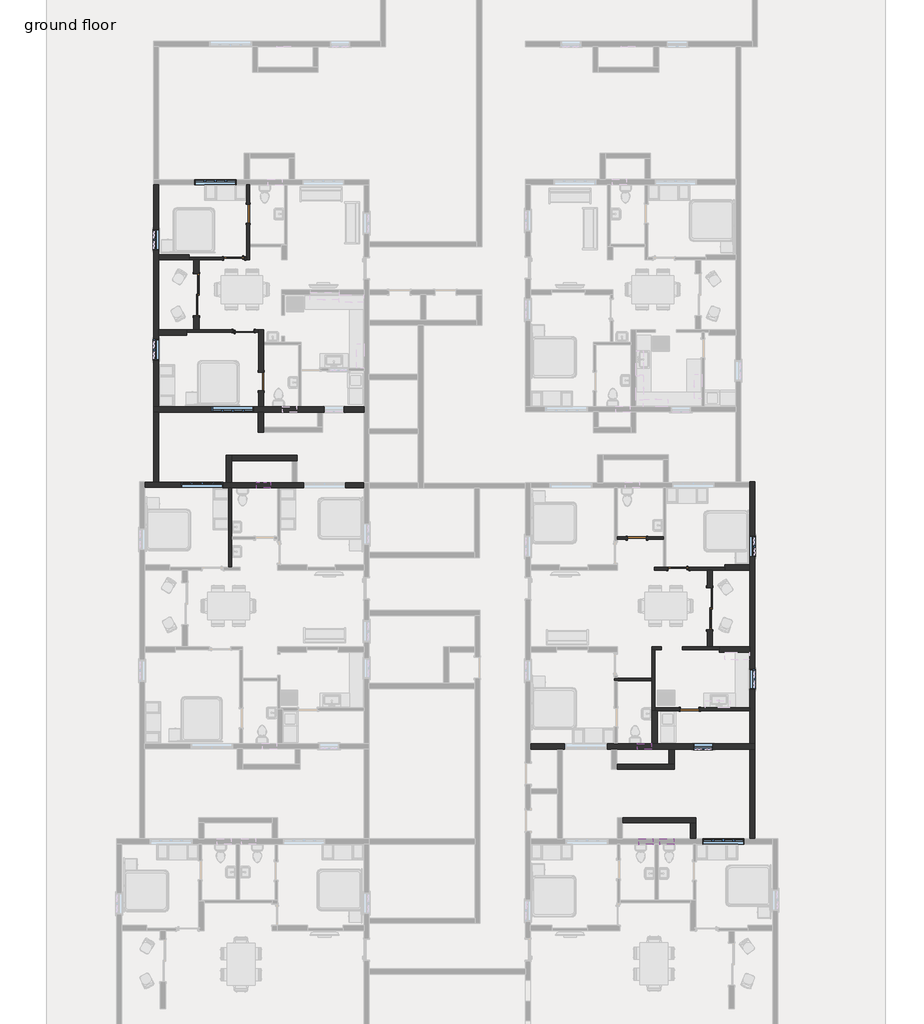
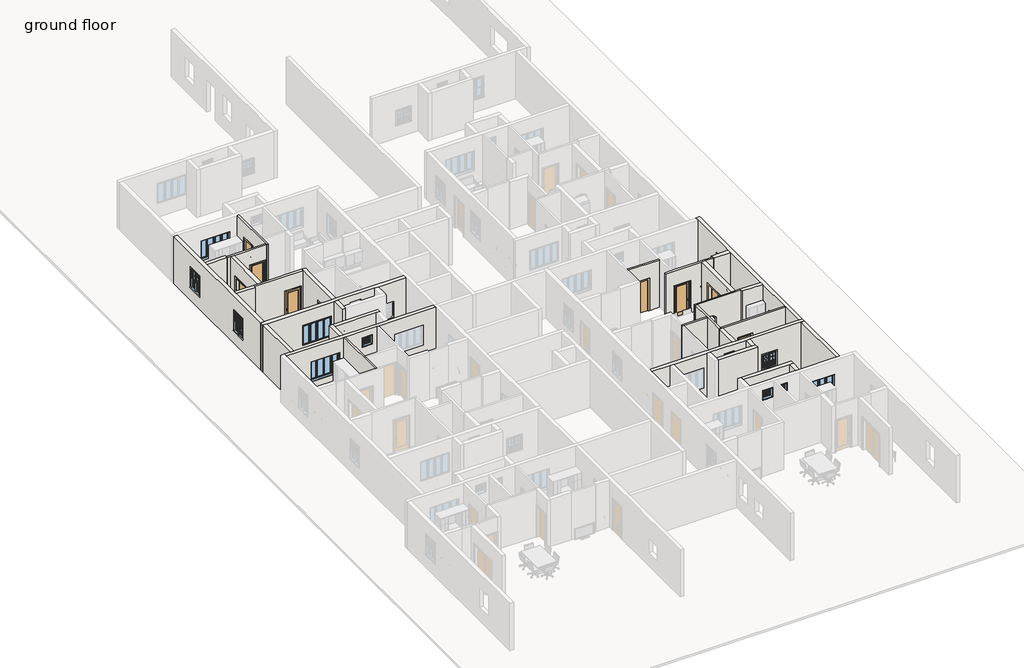
# One storey, part 4 of 16: 32 walls, 13 windows, 9 doors.
# Revit data of these elements (continued)
# Element 42 (IfcWindow, "Window-Casement-Double-Awning : 34\" x 36\"")
#   Mark = "76"
#   Window Inset = 0' - 0"
#   Interior Wall Closure = 0' - 2 1/4"
#   Frame Extension = 0' - 0 1/4"
#   Exterior Wall Closure = 0' - 1 1/4"
#   Interior Trim Visibility = yes
#   Exterior Trim Visibility = yes
#   Phase Created = New Construction
#   Materials on its faces: "Wood - Stained", "Glass", "Clad - White"
# Element 43 (IfcWindow, "Window-Casement-Double-Awning : 34\" x 36\"")
#   Mark = "77"
#   Window Inset = 0' - 0"
#   Interior Wall Closure = 0' - 2 1/4"
#   Frame Extension = 0' - 0 1/4"
#   Exterior Wall Closure = 0' - 1 1/4"
#   Interior Trim Visibility = yes
#   Exterior Trim Visibility = yes
#   Phase Created = New Construction
#   Materials on its faces: "Wood - Stained", "Glass", "Clad - White"
# Element 44 (IfcWindow, "Window-Casement-Multi-Sash-Horizontal : 72\" x 53\"")
#   Mark = "30"
#   Window Inset = 0' - 0 5/8"
#   Frame Gap 3 = 0' - 1 83/128"
#   Frame Gap 2 = 0' - 0 5/8"
#   Phase Created = New Construction
#   Materials on its faces: "Metal - Aluminum", "Glass"
# Element 45 (IfcWindow, "Window-Casement-Multi-Sash-Horizontal : 72\" x 53\"")
#   Mark = "35"
#   Window Inset = 0' - 0 5/8"
#   Frame Gap 3 = 0' - 1 83/128"
#   Frame Gap 2 = 0' - 0 5/8"
#   Phase Created = New Construction
#   Materials on its faces: "Metal - Aluminum", "Glass"
# Element 46 (IfcWindow, "Window-Casement-Multi-Sash-Horizontal : 72\" x 53\"")
#   Mark = "37"
#   Window Inset = 0' - 0 5/8"
#   Frame Gap 3 = 0' - 1 83/128"
#   Frame Gap 2 = 0' - 0 5/8"
#   Phase Created = New Construction
#   Materials on its faces: "Metal - Aluminum", "Glass"
# Element 47 (IfcWindow, "Window-Casement-Multi-Sash-Horizontal : 72\" x 53\"")
#   Mark = "38"
#   Window Inset = 0' - 0 5/8"
#   Frame Gap 3 = 0' - 1 83/128"
#   Frame Gap 2 = 0' - 0 5/8"
#   Phase Created = New Construction
#   Materials on its faces: "Metal - Aluminum", "Glass"
# Element 48 (IfcWindow, "Window-Louvers : 24\" x 24\"")
#   Mark = "99"
#   Blade Width = 1' - 10 1/2"
#   Phase Created = New Construction
#   Materials on its faces: "Birch"
# Element 49 (IfcWindow, "Window-Louvers : 24\" x 24\"")
#   Mark = "100"
#   Blade Width = 1' - 10 1/2"
#   Phase Created = New Construction
#   Materials on its faces: "Birch"
# Element 50 (IfcWindow, "Window-Louvers : 24\" x 24\"")
#   Mark = "101"
#   Blade Width = 1' - 10 1/2"
#   Phase Created = New Construction
#   Materials on its faces: "Birch"
# Element 51 (IfcWindow, "Window-Louvers : 24\" x 24\"")
#   Mark = "107"
#   Blade Width = 1' - 10 1/2"
#   Phase Created = New Construction
#   Materials on its faces: "Birch"
# Element 52 (IfcWindow, "Window-Single-Hung-Double : 36\" x 52\"")
#   Mark = "50"
#   Window Inset = 0' - 0"
#   Interior Wall Closure = 0' - 1 1/2"
#   Frame Extension = 0' - 1 1/4"
#   Exterior Wall Closure = 0' - 0 1/2"
#   Interior Trim Visibility = yes
#   Indicator Visibility = yes
#   Exterior Trim Visibility = yes
#   Phase Created = New Construction
#   Materials on its faces: "Wood - Stained", "Glass", "Clad - White"
# Element 53 (IfcWindow, "Window-Single-Hung-Double : 36\" x 52\"")
#   Mark = "61"
#   Window Inset = 0' - 0"
#   Interior Wall Closure = 0' - 1 1/2"
#   Frame Extension = 0' - 1 1/4"
#   Exterior Wall Closure = 0' - 0 1/2"
#   Interior Trim Visibility = yes
#   Indicator Visibility = yes
#   Exterior Trim Visibility = yes
#   Phase Created = New Construction
#   Materials on its faces: "Wood - Stained", "Glass", "Clad - White"
# Element 54 (IfcWindow, "Window-Single-Hung-Double : 36\" x 52\"")
#   Mark = "63"
#   Window Inset = 0' - 0"
#   Interior Wall Closure = 0' - 1 1/2"
#   Frame Extension = 0' - 1 1/4"
#   Exterior Wall Closure = 0' - 0 1/2"
#   Interior Trim Visibility = yes
#   Indicator Visibility = yes
#   Exterior Trim Visibility = yes
#   Phase Created = New Construction
#   Materials on its faces: "Wood - Stained", "Glass", "Clad - White"
# Materials
#   "Glass": class "Glass", colour RGB 0 128 192, transparency 0.75, Description = "Soda Lime Glass", Cost = 0
#   "Wood - Birch - Solid Stained Light Low Gloss": class "Wood", colour RGB 210 159 95, transparency 0, Cost = 0
#   "Paint - Sienna": colour RGB 118 70 51, transparency 0, Cost = 0
#   "Cherry": class "Wood", colour RGB 226 177 128, transparency 0, Description = "Prunus Serotina", Cost = 0
#   "Aluminum": class "Metal", colour RGB 247 247 247, transparency 0, Description = "Aluminum 6061", Cost = 0
#   "Door - Panel": class "Wood", colour RGB 210 159 95, transparency 0, Cost = 0
#   "Door - Frame": colour RGB 118 70 51, transparency 0, Cost = 0
#   "Wood - Stained": class "Wood", colour RGB 224 178 126, transparency 0, Cost = 0
#   "Clad - White": class "Wood", colour RGB 242 242 238, transparency 0, Cost = 0
#   "Metal - Aluminum": class "Metal", colour RGB 247 247 247, transparency 0
#   "Birch": class "Wood", colour RGB 224 178 126, transparency 0, Description = "Betula Alleghaniensis", Cost = 0
#   "Default Wall": colour RGB 128 128 128, transparency 0, Cost = 0
